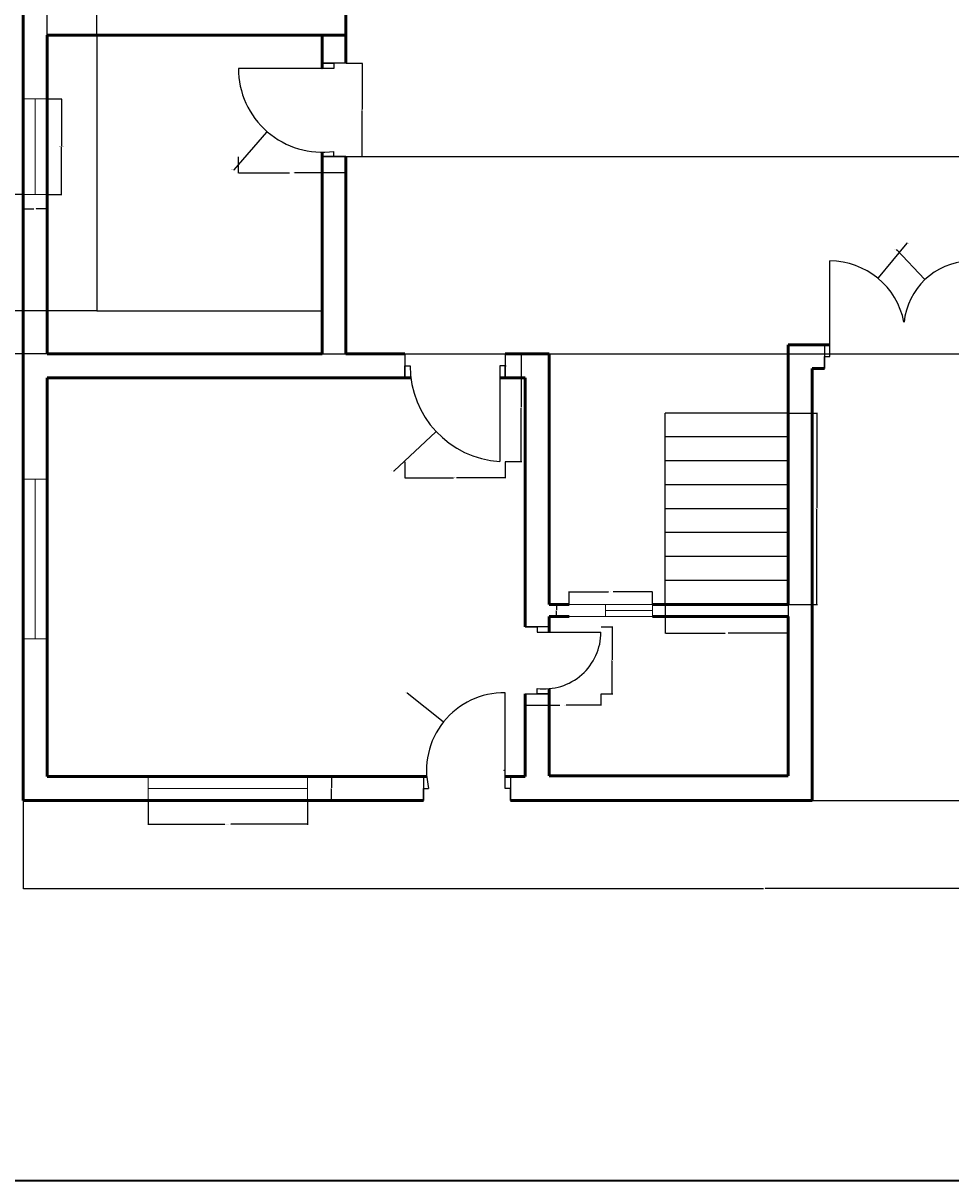
# Model space of a CAD drawing. Units: inches. Extents: x 2215 to 3724, y 1009 to 2124.
# Tile 8 of 11: x 2963 to 3312, y 1009 to 1444. Entities that reach past the tile are written whole.
import ezdxf

# ---------------------------------------------------------------- set-up
doc = ezdxf.new("R2010")
doc.units = ezdxf.units.IN
for name, color, linetype, lineweight in [('A-ANNO-DIMS', 2, 'Continuous', 18), ('A-ANNO-TTLB', 7, 'Continuous', 35), ('A-DOOR', 3, 'Continuous', 25), ('A-FLOR-CASE', 7, 'Continuous', 25), ('A-FLOR-STRS', 7, 'Continuous', 25), ('A-GLAZ', 4, 'Continuous', 18), ('A-WALL', 7, 'Continuous', 50)]:
    doc.layers.add(name, color=color, linetype=linetype, lineweight=lineweight)
doc.styles.get("Standard").update_dxf_attribs({"font": 'arial.ttf'})
doc.dimstyles.get("Standard").update_dxf_attribs({"dimtxt": 0.18, "dimasz": 0.18, "dimexe": 0.18, "dimexo": 0.0625, "dimgap": 0.09, "dimtad": 0, "dimtih": 1, "dimtoh": 1, "dimdec": 4, "dimzin": 0, "dimdsep": 46, "dimtxsty": 'Standard', "dimcen": 0.09, "dimadec": 0, "dimazin": 0, "dimtfac": 1, "dimtdec": 4, "dimtofl": 0, "dimtmove": 0, "dimatfit": 3, "dimfxl": 1, "dimtolj": 1, "dimtzin": 0, "dimarcsym": 0})

# ---------------------------------------------------------------- blocks, each defined once
blk = doc.blocks.new('DOOR-ENTRY-PAIR')
for p, q in [((2, 4.5), (2, 40.5)), ((54.26, 4.5), (54.26, 40.5)), ((0, 9), (0, 0)), ((56.26, 9), (56.26, 0)), ((0, 0), (0, 4.5)), ((0, 4.5), (2, 4.5)), ((56.26, 4.5), (54.26, 4.5))]:
    blk.add_line(p, q)
for centre, radius, start, end in [((2, 12.02), 28.48, 11.0167, 90), ((55.55, 14.8), 25.73, 92.8796, 174.0708)]:
    blk.add_arc(centre, radius, start, end)
blk = doc.blocks.new('DOOR-FRONT-SINGLE')
for p, q in [((30.79, 4.5), (30.79, 40.5)), ((0, 9), (0, 0)), ((32.79, 9), (32.79, 0)), ((0, 0), (0, 4.5)), ((0, 4.5), (2, 4.5)), ((32.79, 4.5), (30.79, 4.5)), ((32.79, 0), (32.79, 4.5))]:
    blk.add_line(p, q)
blk.add_arc((30.39, 11.3), 29.2, 89.2162, 193.4744)
blk = doc.blocks.new('DOOR-KITCHEN')
for p, q in [((40.5, 35.21), (31.5, 35.21)), ((31.5, 35.21), (36, 35.21)), ((36, 35.21), (36, 33.21)), ((36, 33.21), (0, 33.21)), ((36, 0), (36, 2)), ((40.5, 0), (31.5, 0)), ((31.5, 0), (36, 0))]:
    blk.add_line(p, q)
blk.add_arc((31.53, 33.21), 31.53, 180, 278.1525)
blk = doc.blocks.new('DOOR-DRAWING-ROOM')
for p, q in [((0, 40.5), (0, 31.5)), ((37.77, 40.5), (37.77, 31.5)), ((0, 31.5), (0, 36)), ((0, 36), (2, 36)), ((37.77, 36), (35.77, 36)), ((35.77, 36), (35.77, 0)), ((37.77, 31.5), (37.77, 36))]:
    blk.add_line(p, q)
blk.add_arc((38.07, 36), 36.07, 180, 266.3399)
blk = doc.blocks.new('DOOR-BATH-FRONT')
for p, q in [((9, 25.25), (0, 25.25)), ((0, 25.25), (4.5, 25.25)), ((4.5, 25.25), (4.5, 23.25)), ((4.5, 23.25), (28.5, 23.25)), ((4.5, 0), (4.5, 2)), ((0, 0), (9, 0)), ((9, 0), (4.5, 0))]:
    blk.add_line(p, q)
blk.add_arc((7.1, 23.25), 21.4, 263.0342, 0)
blk = doc.blocks.new('WIN-60-JAMB-B')
for p, q in [((9, 60), (0, 60)), ((0, 60), (4.5, 60)), ((4.5, 60), (4.5, 0)), ((4.5, 0), (0, 0)), ((0, 0), (9, 0))]:
    blk.add_line(p, q)
blk = doc.blocks.new('VENT-FRONT-BATH')
for p, q in [((0, 4.5), (31.33, 4.5)), ((13.67, 4.5), (13.67, 4.5)), ((13.67, 4.5), (13.67, 0)), ((31.33, 4.5), (31.33, 0)), ((31.33, 2.25), (13.67, 2.25)), ((0, 0), (0, 0)), ((0, 0), (0, 0)), ((0, 0), (31.33, 0))]:
    blk.add_line(p, q)
blk = doc.blocks.new('WIN-60-FRONT')
for p, q in [((0, 9), (0, 9)), ((0, 9), (0, 0)), ((60, 4.5), (60, 9)), ((60, 9), (60, 0)), ((0, 0), (0, 4.5)), ((0, 4.5), (60, 4.5))]:
    blk.add_line(p, q)
blk = doc.blocks.new('WIN-KITCHEN-36')
for p, q in [((0, 36), (9, 36)), ((9, 36), (4.5, 36)), ((4.5, 36), (4.5, 0)), ((4.5, 0), (0, 0)), ((0, 0), (9, 0))]:
    blk.add_line(p, q)
blk = doc.blocks.new('STAIR-FLIGHT-PLAN')
for p, q in [((0, 0), (0, 72)), ((46.33, 72), (0, 72)), ((46.33, 63), (0, 63)), ((46.33, 54), (0, 54)), ((46.33, 45), (0, 45)), ((46.33, 36), (0, 36)), ((46.33, 27), (0, 27)), ((46.33, 18), (0, 18)), ((46.33, 9), (0, 9))]:
    blk.add_line(p, q)
blk = doc.blocks.new('*D45')
at = {"layer": 'A-ANNO-DIMS', "color": 0, "lineweight": -2, "transparency": 16777216}
for p, q in [((3168.25, 1225.81), (3168.25, 1230.62)), ((3168.43, 1230.44), (3183.02, 1230.44)), ((3199.4, 1230.44), (3184.82, 1230.44)), ((3199.58, 1225.81), (3199.58, 1230.62))]:
    blk.add_line(p, q, dxfattribs=at)
at = {"layer": 'A-ANNO-DIMS', "color": 0, "transparency": 16777216}
for points in [[(3168.43, 1230.47), (3168.43, 1230.41), (3168.25, 1230.44)], [(3199.4, 1230.47), (3199.4, 1230.41), (3199.58, 1230.44)]]:
    blk.add_solid(points, dxfattribs=at)
at = {"layer": 'Defpoints', "color": 0, "transparency": 16777216}
for p in [(3199.58, 1230.44), (3168.25, 1225.74), (3199.58, 1225.74)]:
    blk.add_point(p, dxfattribs=at)
at = {"layer": 'A-ANNO-DIMS', "color": 0, "transparency": 16777216, "insert": (3183.92, 1230.44), "char_height": 0.18, "attachment_point": 5}
blk.add_mtext('\\A1;VENT 31 TYP.', dxfattribs=at)
blk = doc.blocks.new('*D46')
at = {"layer": 'A-ANNO-DIMS', "color": 0, "lineweight": -2, "transparency": 16777216}
for p, q in [((3168.19, 1225.74), (3163.38, 1225.74)), ((3163.56, 1225.56), (3163.56, 1223.68)), ((3168.19, 1221.24), (3163.38, 1221.24)), ((3163.56, 1221.42), (3163.56, 1223.31))]:
    blk.add_line(p, q, dxfattribs=at)
at = {"layer": 'A-ANNO-DIMS', "color": 0, "transparency": 16777216}
for points in [[(3163.53, 1225.56), (3163.59, 1225.56), (3163.56, 1225.74)], [(3163.53, 1221.42), (3163.59, 1221.42), (3163.56, 1221.24)]]:
    blk.add_solid(points, dxfattribs=at)
at = {"layer": 'Defpoints', "color": 0, "transparency": 16777216}
for p in [(3163.56, 1225.74), (3168.25, 1225.74), (3168.25, 1221.24)]:
    blk.add_point(p, dxfattribs=at)
at = {"layer": 'A-ANNO-DIMS', "color": 0, "transparency": 16777216, "insert": (3163.56, 1223.49), "char_height": 0.18, "attachment_point": 5}
blk.add_mtext('\\A1;5 TYP.', dxfattribs=at)
blk = doc.blocks.new('*D47')
at = {"layer": 'A-ANNO-DIMS', "color": 0, "lineweight": -2, "transparency": 16777216}
for p, q in [((3009.8, 1151.93), (3009.8, 1142.82)), ((3069.8, 1151.93), (3069.8, 1142.82)), ((3009.98, 1143), (3038.69, 1143)), ((3069.62, 1143), (3040.92, 1143))]:
    blk.add_line(p, q, dxfattribs=at)
at = {"layer": 'A-ANNO-DIMS', "color": 0, "transparency": 16777216}
for points in [[(3009.98, 1143.03), (3009.98, 1142.97), (3009.8, 1143)], [(3069.62, 1143.03), (3069.62, 1142.97), (3069.8, 1143)]]:
    blk.add_solid(points, dxfattribs=at)
at = {"layer": 'Defpoints', "color": 0, "transparency": 16777216}
for p in [(3009.8, 1152), (3069.8, 1152), (3069.8, 1143)]:
    blk.add_point(p, dxfattribs=at)
at = {"layer": 'A-ANNO-DIMS', "color": 0, "transparency": 16777216, "insert": (3039.8, 1143), "char_height": 0.18, "attachment_point": 5}
blk.add_mtext('\\A1;WINDOW 60 TYP.', dxfattribs=at)
blk = doc.blocks.new('*D48')
at = {"layer": 'A-ANNO-DIMS', "color": 0, "lineweight": -2, "transparency": 16777216}
for p, q in [((3069.87, 1161), (3078.98, 1161)), ((3078.8, 1160.82), (3078.8, 1156.68)), ((3078.8, 1152.18), (3078.8, 1156.32)), ((3069.87, 1152), (3078.98, 1152))]:
    blk.add_line(p, q, dxfattribs=at)
at = {"layer": 'A-ANNO-DIMS', "color": 0, "transparency": 16777216}
for points in [[(3078.77, 1160.82), (3078.83, 1160.82), (3078.8, 1161)], [(3078.77, 1152.18), (3078.83, 1152.18), (3078.8, 1152)]]:
    blk.add_solid(points, dxfattribs=at)
at = {"layer": 'Defpoints', "color": 0, "transparency": 16777216}
for p in [(3069.8, 1161), (3078.8, 1161), (3069.8, 1152)]:
    blk.add_point(p, dxfattribs=at)
at = {"layer": 'A-ANNO-DIMS', "color": 0, "transparency": 16777216, "insert": (3078.8, 1156.5), "char_height": 0.18, "attachment_point": 5}
blk.add_mtext('\\A1;9 TYP.', dxfattribs=at)
blk = doc.blocks.new('*D51')
at = {"layer": 'A-ANNO-DIMS', "color": 0, "lineweight": -2, "transparency": 16777216}
for p, q in [((2971.81, 1416.03), (2977.32, 1416.03)), ((2977.14, 1415.85), (2977.14, 1398.21)), ((2977.14, 1380.21), (2977.14, 1397.85)), ((2971.81, 1380.03), (2977.32, 1380.03))]:
    blk.add_line(p, q, dxfattribs=at)
at = {"layer": 'A-ANNO-DIMS', "color": 0, "transparency": 16777216}
for points in [[(2977.11, 1415.85), (2977.17, 1415.85), (2977.14, 1416.03)], [(2977.11, 1380.21), (2977.17, 1380.21), (2977.14, 1380.03)]]:
    blk.add_solid(points, dxfattribs=at)
at = {"layer": 'Defpoints', "color": 0, "transparency": 16777216}
for p in [(2971.74, 1416.03), (2977.14, 1416.03), (2971.74, 1380.03)]:
    blk.add_point(p, dxfattribs=at)
at = {"layer": 'A-ANNO-DIMS', "color": 0, "transparency": 16777216, "insert": (2977.14, 1398.03), "char_height": 0.18, "attachment_point": 5}
blk.add_mtext('\\A1;WINDOW 36 TYP.', dxfattribs=at)
blk = doc.blocks.new('*D52')
at = {"layer": 'A-ANNO-DIMS', "color": 0, "lineweight": -2, "transparency": 16777216}
for p, q in [((2962.74, 1379.97), (2962.74, 1374.45)), ((2971.74, 1379.97), (2971.74, 1374.45)), ((2962.92, 1374.63), (2966.79, 1374.63)), ((2971.56, 1374.63), (2967.7, 1374.63))]:
    blk.add_line(p, q, dxfattribs=at)
at = {"layer": 'A-ANNO-DIMS', "color": 0, "transparency": 16777216}
for points in [[(2962.92, 1374.66), (2962.92, 1374.6), (2962.74, 1374.63)], [(2971.56, 1374.66), (2971.56, 1374.6), (2971.74, 1374.63)]]:
    blk.add_solid(points, dxfattribs=at)
at = {"layer": 'Defpoints', "color": 0, "transparency": 16777216}
for p in [(2962.74, 1380.03), (2971.74, 1380.03), (2971.74, 1374.63)]:
    blk.add_point(p, dxfattribs=at)
at = {"layer": 'A-ANNO-DIMS', "color": 0, "transparency": 16777216, "insert": (2967.24, 1374.63), "char_height": 0.18, "attachment_point": 5}
blk.add_mtext('\\A1;9 TYP.', dxfattribs=at)
blk = doc.blocks.new('*D69')
at = {"layer": 'A-ANNO-DIMS', "color": 0, "lineweight": -2, "transparency": 16777216}
for p, q in [((3043.74, 1394.19), (3043.74, 1388)), ((3084.24, 1394.19), (3084.24, 1388)), ((3043.92, 1388.18), (3063.06, 1388.18)), ((3084.06, 1388.18), (3064.93, 1388.18))]:
    blk.add_line(p, q, dxfattribs=at)
at = {"layer": 'A-ANNO-DIMS', "color": 0, "transparency": 16777216}
for points in [[(3043.92, 1388.21), (3043.92, 1388.15), (3043.74, 1388.18)], [(3084.06, 1388.21), (3084.06, 1388.15), (3084.24, 1388.18)]]:
    blk.add_solid(points, dxfattribs=at)
at = {"layer": 'Defpoints', "color": 0, "transparency": 16777216}
for p in [(3043.74, 1394.25), (3084.24, 1394.25), (3084.24, 1388.18)]:
    blk.add_point(p, dxfattribs=at)
at = {"layer": 'A-ANNO-DIMS', "color": 0, "transparency": 16777216, "insert": (3063.99, 1388.18), "char_height": 0.18, "attachment_point": 5}
blk.add_mtext('\\A1;DOOR 41 TYP.', dxfattribs=at)
blk = doc.blocks.new('*D70')
at = {"layer": 'A-ANNO-DIMS', "color": 0, "lineweight": -2, "transparency": 16777216}
for p, q in [((3084.31, 1429.47), (3090.5, 1429.47)), ((3090.32, 1429.29), (3090.32, 1412.04)), ((3090.32, 1394.43), (3090.32, 1411.68)), ((3084.31, 1394.25), (3090.5, 1394.25))]:
    blk.add_line(p, q, dxfattribs=at)
at = {"layer": 'A-ANNO-DIMS', "color": 0, "transparency": 16777216}
for points in [[(3090.29, 1429.29), (3090.35, 1429.29), (3090.32, 1429.47)], [(3090.29, 1394.43), (3090.35, 1394.43), (3090.32, 1394.25)]]:
    blk.add_solid(points, dxfattribs=at)
at = {"layer": 'Defpoints', "color": 0, "transparency": 16777216}
for p in [(3084.24, 1429.47), (3090.32, 1429.47), (3084.24, 1394.25)]:
    blk.add_point(p, dxfattribs=at)
at = {"layer": 'A-ANNO-DIMS', "color": 0, "transparency": 16777216, "insert": (3090.32, 1411.86), "char_height": 0.18, "attachment_point": 5}
blk.add_mtext('\\A1;35 TYP.', dxfattribs=at)
blk = doc.blocks.new('*D71')
at = {"layer": 'A-ANNO-DIMS', "color": 0, "lineweight": -2, "transparency": 16777216}
for p, q in [((3144.24, 1320), (3150.43, 1320)), ((3150.25, 1319.82), (3150.25, 1299.93)), ((3150.25, 1279.68), (3150.25, 1299.56)), ((3144.24, 1279.5), (3150.43, 1279.5))]:
    blk.add_line(p, q, dxfattribs=at)
at = {"layer": 'A-ANNO-DIMS', "color": 0, "transparency": 16777216}
for points in [[(3150.22, 1319.82), (3150.28, 1319.82), (3150.25, 1320)], [(3150.22, 1279.68), (3150.28, 1279.68), (3150.25, 1279.5)]]:
    blk.add_solid(points, dxfattribs=at)
at = {"layer": 'Defpoints', "color": 0, "transparency": 16777216}
for p in [(3144.18, 1320), (3150.25, 1320), (3144.18, 1279.5)]:
    blk.add_point(p, dxfattribs=at)
at = {"layer": 'A-ANNO-DIMS', "color": 0, "transparency": 16777216, "insert": (3150.25, 1299.75), "char_height": 0.18, "attachment_point": 5}
blk.add_mtext('\\A1;DOOR 41 TYP.', dxfattribs=at)
blk = doc.blocks.new('*D72')
at = {"layer": 'A-ANNO-DIMS', "color": 0, "lineweight": -2, "transparency": 16777216}
for p, q in [((3106.41, 1279.43), (3106.41, 1273.24)), ((3144.18, 1279.43), (3144.18, 1273.24)), ((3106.59, 1273.42), (3124.76, 1273.42)), ((3144, 1273.42), (3125.82, 1273.42))]:
    blk.add_line(p, q, dxfattribs=at)
at = {"layer": 'A-ANNO-DIMS', "color": 0, "transparency": 16777216}
for points in [[(3106.59, 1273.45), (3106.59, 1273.39), (3106.41, 1273.42)], [(3144, 1273.45), (3144, 1273.39), (3144.18, 1273.42)]]:
    blk.add_solid(points, dxfattribs=at)
at = {"layer": 'Defpoints', "color": 0, "transparency": 16777216}
for p in [(3106.41, 1279.5), (3144.18, 1279.5), (3144.18, 1273.42)]:
    blk.add_point(p, dxfattribs=at)
at = {"layer": 'A-ANNO-DIMS', "color": 0, "transparency": 16777216, "insert": (3125.29, 1273.42), "char_height": 0.18, "attachment_point": 5}
blk.add_mtext('\\A1;38 TYP.', dxfattribs=at)
blk = doc.blocks.new('*D73')
at = {"layer": 'A-ANNO-DIMS', "color": 0, "lineweight": -2, "transparency": 16777216}
for p, q in [((3151.74, 1192.03), (3151.74, 1187.63)), ((3180.24, 1192.03), (3180.24, 1187.63)), ((3151.92, 1187.81), (3164.8, 1187.81)), ((3180.06, 1187.81), (3167.18, 1187.81))]:
    blk.add_line(p, q, dxfattribs=at)
at = {"layer": 'A-ANNO-DIMS', "color": 0, "transparency": 16777216}
for points in [[(3151.92, 1187.84), (3151.92, 1187.78), (3151.74, 1187.81)], [(3180.06, 1187.84), (3180.06, 1187.78), (3180.24, 1187.81)]]:
    blk.add_solid(points, dxfattribs=at)
at = {"layer": 'Defpoints', "color": 0, "transparency": 16777216}
for p in [(3151.74, 1192.09), (3180.24, 1192.09), (3180.24, 1187.81)]:
    blk.add_point(p, dxfattribs=at)
at = {"layer": 'A-ANNO-DIMS', "color": 0, "transparency": 16777216, "insert": (3165.99, 1187.81), "char_height": 0.18, "attachment_point": 5}
blk.add_mtext('\\A1;WC DOOR 29 TYP.', dxfattribs=at)
blk = doc.blocks.new('*D74')
at = {"layer": 'A-ANNO-DIMS', "color": 0, "lineweight": -2, "transparency": 16777216}
for p, q in [((3180.31, 1217.34), (3184.7, 1217.34)), ((3184.52, 1217.16), (3184.52, 1204.89)), ((3184.52, 1192.27), (3184.52, 1204.53)), ((3180.31, 1192.09), (3184.7, 1192.09))]:
    blk.add_line(p, q, dxfattribs=at)
at = {"layer": 'A-ANNO-DIMS', "color": 0, "transparency": 16777216}
for points in [[(3184.49, 1217.16), (3184.55, 1217.16), (3184.52, 1217.34)], [(3184.49, 1192.27), (3184.55, 1192.27), (3184.52, 1192.09)]]:
    blk.add_solid(points, dxfattribs=at)
at = {"layer": 'Defpoints', "color": 0, "transparency": 16777216}
for p in [(3180.24, 1217.34), (3184.52, 1217.34), (3180.24, 1192.09)]:
    blk.add_point(p, dxfattribs=at)
at = {"layer": 'A-ANNO-DIMS', "color": 0, "transparency": 16777216, "insert": (3184.52, 1204.71), "char_height": 0.18, "attachment_point": 5}
blk.add_mtext('\\A1;25 TYP.', dxfattribs=at)
blk = doc.blocks.new('*D75')
at = {"layer": 'A-ANNO-DIMS', "color": 0, "lineweight": -2, "transparency": 16777216}
for p, q in [((3250.81, 1297.74), (3261.72, 1297.74)), ((3261.54, 1297.56), (3261.54, 1261.93)), ((3261.54, 1225.92), (3261.54, 1261.56)), ((3250.81, 1225.74), (3261.72, 1225.74))]:
    blk.add_line(p, q, dxfattribs=at)
at = {"layer": 'A-ANNO-DIMS', "color": 0, "transparency": 16777216}
for points in [[(3261.51, 1297.56), (3261.57, 1297.56), (3261.54, 1297.74)], [(3261.51, 1225.92), (3261.57, 1225.92), (3261.54, 1225.74)]]:
    blk.add_solid(points, dxfattribs=at)
at = {"layer": 'Defpoints', "color": 0, "transparency": 16777216}
for p in [(3250.74, 1297.74), (3261.54, 1297.74), (3250.74, 1225.74)]:
    blk.add_point(p, dxfattribs=at)
at = {"layer": 'A-ANNO-DIMS', "color": 0, "transparency": 16777216, "insert": (3261.54, 1261.74), "char_height": 0.18, "attachment_point": 5}
blk.add_mtext('\\A1;STAIR 72 TYP.', dxfattribs=at)
blk = doc.blocks.new('*D76')
at = {"layer": 'A-ANNO-DIMS', "color": 0, "lineweight": -2, "transparency": 16777216}
for p, q in [((3204.42, 1225.68), (3204.42, 1214.76)), ((3250.74, 1225.68), (3250.74, 1214.76)), ((3204.6, 1214.94), (3227.05, 1214.94)), ((3250.56, 1214.94), (3228.11, 1214.94))]:
    blk.add_line(p, q, dxfattribs=at)
at = {"layer": 'A-ANNO-DIMS', "color": 0, "transparency": 16777216}
for points in [[(3204.6, 1214.97), (3204.6, 1214.91), (3204.42, 1214.94)], [(3250.56, 1214.97), (3250.56, 1214.91), (3250.74, 1214.94)]]:
    blk.add_solid(points, dxfattribs=at)
at = {"layer": 'Defpoints', "color": 0, "transparency": 16777216}
for p in [(3204.42, 1225.74), (3250.74, 1225.74), (3250.74, 1214.94)]:
    blk.add_point(p, dxfattribs=at)
at = {"layer": 'A-ANNO-DIMS', "color": 0, "transparency": 16777216, "insert": (3227.58, 1214.94), "char_height": 0.18, "attachment_point": 5}
blk.add_mtext('\\A1;46 TYP.', dxfattribs=at)
blk = doc.blocks.new('*D90')
at = {"layer": 'A-ANNO-DIMS', "color": 0, "lineweight": -2, "transparency": 16777216}
for p, q in [((2962.68, 1380.03), (2877.61, 1380.03)), ((2877.79, 1379.85), (2877.79, 1350.2)), ((2877.79, 1320.18), (2877.79, 1349.83)), ((2971.68, 1320), (2877.61, 1320))]:
    blk.add_line(p, q, dxfattribs=at)
at = {"layer": 'A-ANNO-DIMS', "color": 0, "transparency": 16777216}
for points in [[(2877.76, 1379.85), (2877.82, 1379.85), (2877.79, 1380.03)], [(2877.76, 1320.18), (2877.82, 1320.18), (2877.79, 1320)]]:
    blk.add_solid(points, dxfattribs=at)
at = {"layer": 'Defpoints', "color": 0, "transparency": 16777216}
for p in [(2877.79, 1380.03), (2962.74, 1380.03), (2971.74, 1320)]:
    blk.add_point(p, dxfattribs=at)
at = {"layer": 'A-ANNO-DIMS', "color": 0, "transparency": 16777216, "insert": (2877.79, 1350.01), "char_height": 0.18, "attachment_point": 5}
blk.add_mtext('\\A1;60.03', dxfattribs=at)
blk = doc.blocks.new('*D96')
at = {"layer": 'A-ANNO-DIMS', "color": 0, "lineweight": -2, "transparency": 16777216}
for p, q in [((3520.74, 1343.93), (3520.74, 1118.67)), ((2962.74, 1151.93), (2962.74, 1118.67)), ((2962.92, 1118.85), (3241.45, 1118.85)), ((3520.56, 1118.85), (3242.03, 1118.85))]:
    blk.add_line(p, q, dxfattribs=at)
at = {"layer": 'A-ANNO-DIMS', "color": 0, "transparency": 16777216}
for points in [[(2962.92, 1118.88), (2962.92, 1118.82), (2962.74, 1118.85)], [(3520.56, 1118.88), (3520.56, 1118.82), (3520.74, 1118.85)]]:
    blk.add_solid(points, dxfattribs=at)
at = {"layer": 'Defpoints', "color": 0, "transparency": 16777216}
for p in [(3520.74, 1344), (2962.74, 1152), (3520.74, 1118.85)]:
    blk.add_point(p, dxfattribs=at)
at = {"layer": 'A-ANNO-DIMS', "color": 0, "transparency": 16777216, "insert": (3241.74, 1118.85), "char_height": 0.18, "attachment_point": 5}
blk.add_mtext('\\A1;558', dxfattribs=at)
blk = doc.blocks.new('*D97')
at = {"layer": 'A-ANNO-DIMS', "color": 0, "lineweight": -2, "transparency": 16777216}
for p, q in [((3520.81, 1747.5), (3590.27, 1747.5)), ((3590.09, 1747.32), (3590.09, 1449.93)), ((3590.09, 1152.18), (3590.09, 1449.57)), ((3259.81, 1152), (3590.27, 1152))]:
    blk.add_line(p, q, dxfattribs=at)
at = {"layer": 'A-ANNO-DIMS', "color": 0, "transparency": 16777216}
for points in [[(3590.06, 1747.32), (3590.12, 1747.32), (3590.09, 1747.5)], [(3590.06, 1152.18), (3590.12, 1152.18), (3590.09, 1152)]]:
    blk.add_solid(points, dxfattribs=at)
at = {"layer": 'Defpoints', "color": 0, "transparency": 16777216}
for p in [(3520.74, 1747.5), (3590.09, 1747.5), (3259.74, 1152)]:
    blk.add_point(p, dxfattribs=at)
at = {"layer": 'A-ANNO-DIMS', "color": 0, "transparency": 16777216, "insert": (3590.09, 1449.75), "char_height": 0.18, "attachment_point": 5}
blk.add_mtext('\\A1;595.5', dxfattribs=at)
blk = doc.blocks.new('*D126')
at = {"layer": 'A-ANNO-DIMS', "color": 0, "lineweight": -2, "transparency": 16777216}
for p, q in [((2990.35, 1336.24), (2877.61, 1336.24)), ((2877.79, 1336.06), (2877.79, 1328.3)), ((2877.79, 1320.18), (2877.79, 1327.94)), ((2971.68, 1320), (2877.61, 1320))]:
    blk.add_line(p, q, dxfattribs=at)
at = {"layer": 'A-ANNO-DIMS', "color": 0, "transparency": 16777216}
for points in [[(2877.76, 1336.06), (2877.82, 1336.06), (2877.79, 1336.24)], [(2877.76, 1320.18), (2877.82, 1320.18), (2877.79, 1320)]]:
    blk.add_solid(points, dxfattribs=at)
at = {"layer": 'Defpoints', "color": 0, "transparency": 16777216}
for p in [(2877.79, 1336.24), (2990.42, 1336.24), (2971.74, 1320)]:
    blk.add_point(p, dxfattribs=at)
at = {"layer": 'A-ANNO-DIMS', "color": 0, "transparency": 16777216, "insert": (2877.79, 1328.12), "char_height": 0.18, "attachment_point": 5}
blk.add_mtext('\\A1;16.24', dxfattribs=at)
blk = doc.blocks.new('*D127')
at = {"layer": 'A-ANNO-DIMS', "color": 0, "lineweight": -2, "transparency": 16777216}
for p, q in [((2971.74, 1440.06), (2971.74, 1780.83)), ((2971.92, 1780.65), (2980.62, 1780.65)), ((2990.24, 1780.65), (2981.53, 1780.65)), ((2990.42, 1440.06), (2990.42, 1780.83))]:
    blk.add_line(p, q, dxfattribs=at)
at = {"layer": 'A-ANNO-DIMS', "color": 0, "transparency": 16777216}
for points in [[(2971.92, 1780.68), (2971.92, 1780.62), (2971.74, 1780.65)], [(2990.24, 1780.68), (2990.24, 1780.62), (2990.42, 1780.65)]]:
    blk.add_solid(points, dxfattribs=at)
at = {"layer": 'Defpoints', "color": 0, "transparency": 16777216}
for p in [(2990.42, 1780.65), (2971.74, 1440), (2990.42, 1440)]:
    blk.add_point(p, dxfattribs=at)
at = {"layer": 'A-ANNO-DIMS', "color": 0, "transparency": 16777216, "insert": (2981.08, 1780.65), "char_height": 0.18, "attachment_point": 5}
blk.add_mtext('\\A1;18.673', dxfattribs=at)
blk = doc.blocks.new('*D128')
at = {"layer": 'A-ANNO-DIMS', "color": 0, "lineweight": -2, "transparency": 16777216}
for p, q in [((3075.31, 1394.25), (3590.27, 1394.25)), ((3590.09, 1394.07), (3590.09, 1357.31)), ((3590.09, 1320.18), (3590.09, 1356.94)), ((3075.31, 1320), (3590.27, 1320))]:
    blk.add_line(p, q, dxfattribs=at)
at = {"layer": 'A-ANNO-DIMS', "color": 0, "transparency": 16777216}
for points in [[(3590.06, 1394.07), (3590.12, 1394.07), (3590.09, 1394.25)], [(3590.06, 1320.18), (3590.12, 1320.18), (3590.09, 1320)]]:
    blk.add_solid(points, dxfattribs=at)
at = {"layer": 'Defpoints', "color": 0, "transparency": 16777216}
for p in [(3075.24, 1394.25), (3590.09, 1394.25), (3075.24, 1320)]:
    blk.add_point(p, dxfattribs=at)
at = {"layer": 'A-ANNO-DIMS', "color": 0, "transparency": 16777216, "insert": (3590.09, 1357.13), "char_height": 0.18, "attachment_point": 5}
blk.add_mtext('\\A1;74.26', dxfattribs=at)
blk = doc.blocks.new('*D132')
at = {"layer": 'A-ANNO-DIMS', "color": 0, "lineweight": -2, "transparency": 16777216}
for p, q in [((3144.39, 1315.5), (3144.57, 1315.5)), ((3144.48, 1315.41), (3144.48, 1315.59)), ((3102.38, 1276.01), (3118.04, 1290.69)), ((3102.2, 1276.01), (3102.38, 1276.01))]:
    blk.add_line(p, q, dxfattribs=at)
at = {"layer": 'A-ANNO-DIMS', "color": 0, "transparency": 16777216}
blk.add_solid([(3118.02, 1290.72), (3118.06, 1290.67), (3118.17, 1290.82)], dxfattribs=at)
at = {"layer": 'Defpoints', "color": 0, "transparency": 16777216}
for p in [(3144.48, 1315.5), (3118.17, 1290.82)]:
    blk.add_point(p, dxfattribs=at)
at = {"layer": 'A-ANNO-DIMS', "color": 0, "transparency": 16777216, "insert": (3101.73, 1276.01), "char_height": 0.18, "attachment_point": 5}
blk.add_mtext('\\A1;R36.07', dxfattribs=at)
blk = doc.blocks.new('*D134')
at = {"layer": 'A-ANNO-DIMS', "color": 0, "lineweight": -2, "transparency": 16777216}
for p, q in [((3075.18, 1427.47), (3075.36, 1427.47)), ((3075.27, 1427.38), (3075.27, 1427.56)), ((3042.23, 1389.35), (3054.5, 1403.51)), ((3042.05, 1389.35), (3042.23, 1389.35))]:
    blk.add_line(p, q, dxfattribs=at)
at = {"layer": 'A-ANNO-DIMS', "color": 0, "transparency": 16777216}
blk.add_solid([(3054.48, 1403.53), (3054.52, 1403.49), (3054.62, 1403.64)], dxfattribs=at)
at = {"layer": 'Defpoints', "color": 0, "transparency": 16777216}
for p in [(3075.27, 1427.47), (3054.62, 1403.64)]:
    blk.add_point(p, dxfattribs=at)
at = {"layer": 'A-ANNO-DIMS', "color": 0, "transparency": 16777216, "insert": (3041.57, 1389.35), "char_height": 0.18, "attachment_point": 5}
blk.add_mtext('\\A1;R31.53', dxfattribs=at)
blk = doc.blocks.new('*D136')
at = {"layer": 'A-ANNO-DIMS', "color": 0, "lineweight": -2, "transparency": 16777216}
for p, q in [((3107.12, 1192.48), (3107.3, 1192.48)), ((3107.3, 1192.48), (3120.84, 1181.65)), ((3143.78, 1163.21), (3143.78, 1163.39)), ((3143.69, 1163.3), (3143.87, 1163.3))]:
    blk.add_line(p, q, dxfattribs=at)
at = {"layer": 'A-ANNO-DIMS', "color": 0, "transparency": 16777216}
blk.add_solid([(3120.86, 1181.67), (3120.82, 1181.63), (3120.98, 1181.54)], dxfattribs=at)
at = {"layer": 'Defpoints', "color": 0, "transparency": 16777216}
for p in [(3120.98, 1181.54), (3143.78, 1163.3)]:
    blk.add_point(p, dxfattribs=at)
at = {"layer": 'A-ANNO-DIMS', "color": 0, "transparency": 16777216, "insert": (3106.71, 1192.48), "char_height": 0.18, "attachment_point": 5}
blk.add_mtext('\\A1;R29.2', dxfattribs=at)
blk = doc.blocks.new('*D137')
at = {"layer": 'A-ANNO-DIMS', "color": 0, "lineweight": -2, "transparency": 16777216}
for p, q in [((3295.34, 1361.67), (3284.58, 1348.62)), ((3295.52, 1361.67), (3295.34, 1361.67)), ((3266.26, 1326.5), (3266.44, 1326.5)), ((3266.35, 1326.41), (3266.35, 1326.59))]:
    blk.add_line(p, q, dxfattribs=at)
at = {"layer": 'A-ANNO-DIMS', "color": 0, "transparency": 16777216}
blk.add_solid([(3284.56, 1348.64), (3284.61, 1348.6), (3284.47, 1348.48)], dxfattribs=at)
at = {"layer": 'Defpoints', "color": 0, "transparency": 16777216}
for p in [(3284.47, 1348.48), (3266.35, 1326.5)]:
    blk.add_point(p, dxfattribs=at)
at = {"layer": 'A-ANNO-DIMS', "color": 0, "transparency": 16777216, "insert": (3296.07, 1361.67), "char_height": 0.18, "attachment_point": 5}
blk.add_mtext('\\A1;R28.484', dxfattribs=at)
blk = doc.blocks.new('*D138')
at = {"layer": 'A-ANNO-DIMS', "color": 0, "lineweight": -2, "transparency": 16777216}
for p, q in [((3291.4, 1359.16), (3291.58, 1359.16)), ((3291.58, 1359.16), (3302.08, 1348.09)), ((3319.82, 1329.29), (3320, 1329.29)), ((3319.91, 1329.2), (3319.91, 1329.38))]:
    blk.add_line(p, q, dxfattribs=at)
at = {"layer": 'A-ANNO-DIMS', "color": 0, "transparency": 16777216}
blk.add_solid([(3302.1, 1348.11), (3302.06, 1348.07), (3302.2, 1347.96)], dxfattribs=at)
at = {"layer": 'Defpoints', "color": 0, "transparency": 16777216}
for p in [(3302.2, 1347.96), (3319.91, 1329.29)]:
    blk.add_point(p, dxfattribs=at)
at = {"layer": 'A-ANNO-DIMS', "color": 0, "transparency": 16777216, "insert": (3290.92, 1359.16), "char_height": 0.18, "attachment_point": 5}
blk.add_mtext('\\A1;R25.73', dxfattribs=at)

msp = doc.modelspace()

# ---------------------------------------------------------------- linework, layer by layer
at = {"layer": 'A-ANNO-TTLB'}
msp.add_lwpolyline([(2215.4438, 2124.2681), (3723.6589, 2124.2681), (3723.6589, 1008.7935), (2215.4438, 1008.7935)], close=True, dxfattribs=at)
at = {"layer": 'A-FLOR-CASE'}
for p, q in [((2990.4162, 1439.9969), (2990.4162, 1336.2381)), ((2990.4162, 1336.2381), (3075.2432, 1336.2381))]:
    msp.add_line(p, q, dxfattribs=at)
at = {"layer": 'A-WALL'}
for p, q in [((2962.7432, 1517.9969), (2962.7432, 1151.9969)), ((3084.2432, 1448.9969), (3084.2432, 1429.4651)), ((2971.7432, 1439.9969), (2971.7432, 1319.9969)), ((3084.2432, 1439.9969), (2971.7432, 1439.9969)), ((3075.2432, 1427.4651), (3075.2432, 1439.9969)), ((3075.2432, 1319.9969), (3075.2432, 1395.9362)), ((3084.2432, 1394.2548), (3084.2432, 1319.9969)), ((3250.7432, 1225.7439), (3250.7432, 1323.4864)), ((3250.7432, 1323.4864), (3259.7432, 1323.4864)), ((3259.7432, 1323.4864), (3266.3548, 1323.4864)), ((3075.2432, 1319.9969), (2971.7432, 1319.9969)), ((3106.4066, 1319.9969), (3084.2432, 1319.9969)), ((3160.7432, 1319.9969), (3144.1773, 1319.9969)), ((3151.7432, 1319.9969), (3160.7432, 1319.9969)), ((3160.7432, 1319.9969), (3160.7432, 1225.7439)), ((3259.7432, 1314.4864), (3259.7432, 1160.9969)), ((3264.3548, 1314.4864), (3259.7432, 1314.4864)), ((2971.7432, 1310.9969), (2971.7432, 1160.9969)), ((3108.6883, 1310.9969), (2971.7432, 1310.9969)), ((3151.7432, 1310.9969), (3142.1773, 1310.9969)), ((3151.7432, 1217.3361), (3151.7432, 1310.9969)), ((3168.2546, 1225.7439), (3160.7432, 1225.7439)), ((3250.7432, 1225.7439), (3199.5816, 1225.7439)), ((3160.7432, 1221.2439), (3160.7432, 1215.3361)), ((3160.7432, 1215.3361), (3160.7432, 1221.2439)), ((3160.7432, 1221.2439), (3168.2546, 1221.2439)), ((3199.5816, 1221.2439), (3250.7432, 1221.2439)), ((3250.7432, 1161.2439), (3250.7432, 1221.2439)), ((3160.7432, 1194.0167), (3160.7432, 1161.2439)), ((3160.7432, 1161.2439), (3160.7432, 1194.0167)), ((3151.7432, 1160.9969), (3151.7432, 1192.0899)), ((3114.6721, 1160.9969), (2971.7432, 1160.9969)), ((3151.7432, 1160.9969), (3144.1795, 1160.9969)), ((3160.7432, 1161.2439), (3250.7432, 1161.2439)), ((3259.7432, 1160.9969), (3259.7432, 1151.9969)), ((2962.7432, 1151.9969), (3113.3848, 1151.9969)), ((3113.3848, 1151.9969), (2971.7432, 1151.9969)), ((3160.7432, 1151.9969), (3146.1795, 1151.9969)), ((3146.1795, 1151.9969), (3151.7432, 1151.9969)), ((3160.7432, 1151.9969), (3250.7432, 1151.9969)), ((3259.7432, 1151.9969), (3250.7432, 1151.9969)), ((3250.7432, 1151.9969), (3259.7432, 1151.9969))]:
    msp.add_line(p, q, dxfattribs=at)

# ---------------------------------------------------------------- block references
at = {"layer": 'A-DOOR'}
for name, p in [('DOOR-KITCHEN', (3043.7432, 1394.255)), ('DOOR-ENTRY-PAIR', (3264.3552, 1314.486)), ('DOOR-DRAWING-ROOM', (3106.4062, 1279.497)), ('DOOR-BATH-FRONT', (3151.7432, 1192.09)), ('DOOR-FRONT-SINGLE', (3113.3852, 1151.997))]:
    msp.add_blockref(name, p, dxfattribs=at)
at = {"layer": 'A-FLOR-STRS'}
msp.add_blockref('STAIR-FLIGHT-PLAN', (3204.4152, 1225.744), dxfattribs=at)
at = {"layer": 'A-GLAZ'}
for name, p in [('WIN-KITCHEN-36', (2962.7432, 1380.031)), ('WIN-60-JAMB-B', (2962.7432, 1212.834)), ('VENT-FRONT-BATH', (3168.2542, 1221.244)), ('WIN-60-FRONT', (3009.8052, 1151.997))]:
    msp.add_blockref(name, p, dxfattribs=at)

# ---------------------------------------------------------------- dimensions: what is measured, and where the dimension line sits
at = {"layer": 'A-ANNO-DIMS'}
for base, p1, p2, override, picture, middle in [((2990.4162, 1780.6469), (2971.7432, 1439.9969), (2990.4162, 1439.9969), {"dimdec": 3, "dimlfac": 1, "dimrnd": 0, "dimzin": 0, "dimdsep": 46, "dimlunit": 2}, '*D127', (2981.0797, 1780.6469)), ((3520.7432, 1118.8469), (2962.7432, 1151.9969), (3520.7432, 1343.9969), {"dimdec": 0, "dimlfac": 1, "dimrnd": 0, "dimzin": 0, "dimdsep": 46, "dimlunit": 2}, '*D96', (3241.7432, 1118.8469))]:
    dim = msp.add_linear_dim(base=base, p1=p1, p2=p2, dimstyle='Standard', override=override, dxfattribs=at)
    dim.commit()
    dim.dimension.update_dxf_attribs({"geometry": picture, "text_midpoint": middle})
for base, p1, p2, override, picture, middle in [((3590.0929, 1747.4969), (3259.7432, 1151.9969), (3520.7432, 1747.4969), {"dimdec": 1, "dimlfac": 1, "dimrnd": 0, "dimzin": 0, "dimdsep": 46, "dimlunit": 2}, '*D97', (3590.0929, 1449.7469)), ((3590.0929, 1394.2548), (3075.2432, 1319.9969), (3075.2432, 1394.2548), {"dimdec": 2, "dimlfac": 1, "dimrnd": 0, "dimzin": 0, "dimdsep": 46, "dimlunit": 2}, '*D128', (3590.0929, 1357.1259)), ((2877.7914, 1380.0306), (2971.7432, 1319.9969), (2962.7432, 1380.0306), {"dimdec": 2, "dimlfac": 1, "dimrnd": 0, "dimzin": 0, "dimdsep": 46, "dimlunit": 2}, '*D90', (2877.7914, 1350.0138)), ((2877.7914, 1336.2381), (2971.7432, 1319.9969), (2990.4162, 1336.2381), {"dimdec": 2, "dimlfac": 1, "dimrnd": 0, "dimzin": 0, "dimdsep": 46, "dimlunit": 2}, '*D126', (2877.7914, 1328.1175))]:
    dim = msp.add_linear_dim(base=base, p1=p1, p2=p2, angle=90, dimstyle='Standard', override=override, dxfattribs=at)
    dim.commit()
    dim.dimension.update_dxf_attribs({"geometry": picture, "text_midpoint": middle})
for base, p1, p2, text, picture, middle in [((3090.3182, 1429.4651), (3084.2432, 1394.2548), (3084.2432, 1429.4651), '<> TYP.', '*D70', (3090.3182, 1411.8599)), ((2977.1432, 1416.0306), (2971.7432, 1380.0306), (2971.7432, 1416.0306), 'WINDOW <> TYP.', '*D51', (2977.1432, 1398.0306)), ((3150.2523306975, 1319.9969403012), (3144.1773306975, 1279.4969403012), (3144.1773306975, 1319.9969403012), 'DOOR <> TYP.', '*D71', (3150.2523306975, 1299.7469403012)), ((3261.5432, 1297.7439), (3250.7432, 1225.7439), (3250.7432, 1297.7439), 'STAIR <> TYP.', '*D75', (3261.5432, 1261.7439)), ((3163.5554891558, 1225.7438653031), (3168.254550954, 1221.2438653031), (3168.254550954, 1225.7438653031), '<> TYP.', '*D46', (3163.5554891558, 1223.4938653031)), ((3184.5182, 1217.3361), (3180.2432, 1192.0899), (3180.2432, 1217.3361), '<> TYP.', '*D74', (3184.5182, 1204.713)), ((3078.8049, 1160.9969), (3069.8049, 1151.9969), (3069.8049, 1160.9969), '<> TYP.', '*D48', (3078.8049, 1156.4969))]:
    dim = msp.add_linear_dim(base=base, p1=p1, p2=p2, angle=90, text=text, dimstyle='Standard', override={"dimdec": 0, "dimlfac": 1, "dimrnd": 0, "dimzin": 0, "dimdsep": 46, "dimlunit": 2}, dxfattribs=at)
    dim.commit()
    dim.dimension.update_dxf_attribs({"geometry": picture, "text_midpoint": middle})
for center, mpoint, override, picture, middle in [((3075.2721, 1427.4651), (3054.6192, 1403.6422), {"dimdec": 2, "dimlfac": 1, "dimrnd": 0, "dimzin": 0, "dimdsep": 46, "dimlunit": 2}, '*D134', (3041.5676, 1389.3485)), ((3266.35477, 1326.50288), (3284.4692, 1348.48425), {"dimdec": 3, "dimlfac": 1, "dimrnd": 0, "dimzin": 0, "dimdsep": 46, "dimlunit": 2}, '*D137', (3296.06726, 1361.67307)), ((3319.9068, 1329.2879), (3302.2028, 1347.9602), {"dimdec": 2, "dimlfac": 1, "dimrnd": 0, "dimzin": 0, "dimdsep": 46, "dimlunit": 2}, '*D138', (3290.9206, 1359.1636)), ((3144.4801, 1315.4969), (3118.1707, 1290.8167), {"dimdec": 2, "dimlfac": 1, "dimrnd": 0, "dimzin": 0, "dimdsep": 46, "dimlunit": 2}, '*D132', (3101.7252, 1276.0085)), ((3143.7801, 1163.3006), (3120.9779, 1181.5391), {"dimdec": 1, "dimlfac": 1, "dimrnd": 0, "dimzin": 0, "dimdsep": 46, "dimlunit": 2}, '*D136', (3106.7075, 1192.4822))]:
    dim = msp.add_radius_dim(center=center, mpoint=mpoint, dimstyle='Standard', override=override, dxfattribs=at)
    dim.commit()
    dim.dimension.update_dxf_attribs({"geometry": picture, "text_midpoint": middle, "dimtype": 164})
for base, p1, p2, text, picture, middle in [((3084.2432030508, 1388.1797823387), (3043.7432030508, 1394.2547823387), (3084.2432030508, 1394.2547823387), 'DOOR <> TYP.', '*D69', (3063.9932030508, 1388.1797823387)), ((2971.7432, 1374.6306), (2962.7432, 1380.0306), (2971.7432, 1380.0306), '<> TYP.', '*D52', (2967.2432, 1374.6306)), ((3144.1773, 1273.4219), (3106.4066, 1279.4969), (3144.1773, 1279.4969), '<> TYP.', '*D72', (3125.2919, 1273.4219)), ((3199.5816, 1230.4429), (3168.2546, 1225.7439), (3199.5816, 1225.7439), 'VENT <> TYP.', '*D45', (3183.9181, 1230.4429)), ((3250.7432, 1214.9439), (3204.4152, 1225.7439), (3250.7432, 1225.7439), '<> TYP.', '*D76', (3227.5792, 1214.9439)), ((3180.2432030508, 1187.8148563773), (3151.7432030508, 1192.0898563773), (3180.2432030508, 1192.0898563773), 'WC DOOR <> TYP.', '*D73', (3165.9932030508, 1187.8148563773)), ((3069.8049, 1142.9969), (3009.8049, 1151.9969), (3069.8049, 1151.9969), 'WINDOW <> TYP.', '*D47', (3039.8049, 1142.9969))]:
    dim = msp.add_linear_dim(base=base, p1=p1, p2=p2, text=text, dimstyle='Standard', override={"dimdec": 0, "dimlfac": 1, "dimrnd": 0, "dimzin": 0, "dimdsep": 46, "dimlunit": 2}, dxfattribs=at)
    dim.commit()
    dim.dimension.update_dxf_attribs({"geometry": picture, "text_midpoint": middle})

doc.saveas('drawing.dxf')
